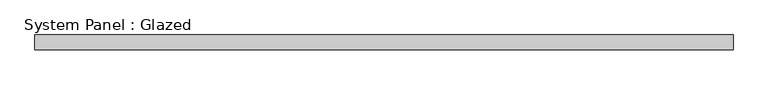
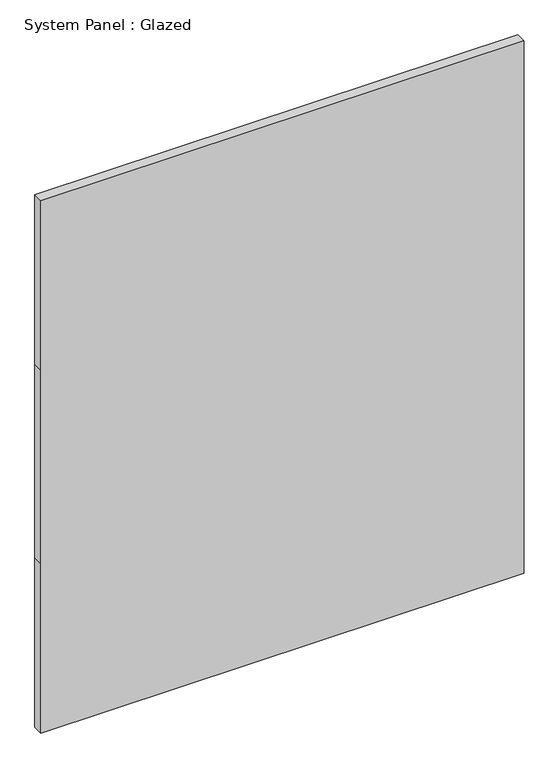
"""IFC4 building model written with IfcOpenShell, lengths in millimetres: plate geometry, System Panel : Glazed."""

from ifc_helpers import new_model, si_unit, frame, origin, place, context, project, spatial, polyline, outline, extrude, source, transform, mapped, element, save


def system_panel_glazed_e5754967(model_context):
    return source(origin(), model_context, "Body", "SweptSolid", [
        extrude(outline(polyline([(0.0, -600.075), (0.0, 600.075), (444.5, 600.075), (952.5, 600.075), (1397.0, 600.075), (1397.0, -600.075), (952.5, -600.075), (444.5, -600.075), (0.0, -600.075)])), frame((0.0, 19.05, 0.0), z_axis=(0.0, 1.0, 0.0), x_axis=(0.0, 0.0, 1.0)), (0.0, 0.0, 1.0), 25.4),
    ])


if __name__ == "__main__":
    model = new_model("IFC4")
    model_context = context("Model", 3, world=origin())
    ifc_project = project(units=[si_unit("LENGTHUNIT", "METRE", prefix="MILLI")], contexts=[model_context])
    site = spatial("IfcSite", under=ifc_project)
    building = spatial("IfcBuilding", under=site)
    placement = place(None, origin())
    system_panel_glazed_shape = system_panel_glazed_e5754967(model_context)
    element("IfcPlate", 1, ObjectType="System Panel : Glazed", at=placement, inside=building, context=model_context, shape_type="MappedRepresentation", body=[
        mapped(system_panel_glazed_shape, transform((0.0, 0.0, 0.0), x_axis=(1.0, 0.0, 0.0), y_axis=(0.0, 1.0, 0.0), z_axis=(0.0, 0.0, 1.0))),
    ])
    save(model, "model.ifc")

# Revit data of these elements
# Type "System Panel : Glazed"
#   Construction Type Id = "GSP4R"
#   Analytic Construction = "1/8 in Pilkington single glazing"
#   Visual Light Transmittance = 0.9
#   Solar Heat Gain Coefficient = 0.86
#   Heat Transfer Coefficient (U) = 1.18115 BTU/(h·ft²·°F)
#   Define Thermal Properties by = 1
# Element 1 (IfcPlate, "System Panel : Glazed")
#   Materials on its faces: "Glass"
# Materials
#   "Glass": class "Glass", colour RGB 0 128 192, transparency 0.75, Description = "Soda Lime Glass", Cost = 0
